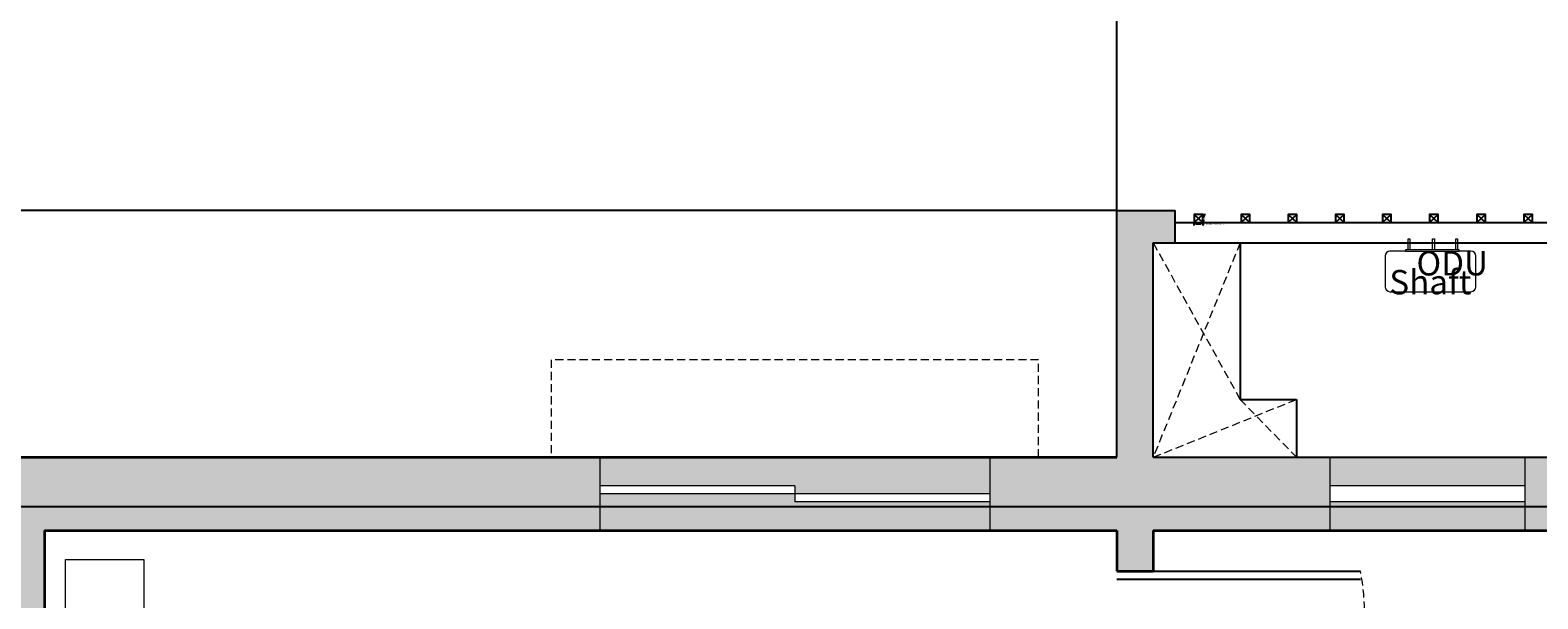
# Model space of a CAD drawing. Units: inches. Extents: x 1693 to 2974, y 2201 to 2965.
# Tile 6 of 24: x 1790 to 1976, y 2689 to 2759. Entities that reach past the tile are written whole.
import ezdxf

# ---------------------------------------------------------------- set-up
doc = ezdxf.new("R2010")
doc.units = ezdxf.units.IN
doc.header["$LTSCALE"] = 2
doc.header["$MEASUREMENT"] = 0
doc.linetypes.add('HIDDEN', pattern=[0.375, 0.25, -0.125])
for name, color, linetype, lineweight in [('A-ANNO-DIMS', 2, 'Continuous', 18), ('A-ANNO-TEXT', 7, 'Continuous', 13), ('A-DOOR', 3, 'Continuous', 25), ('A-DOOR-SWNG', 3, 'HIDDEN', 13), ('A-FLOR-SHFT', 7, 'Continuous', 25), ('A-FLOR-SHFT-HIDN', 8, 'HIDDEN', 13), ('A-FURN', 8, 'Continuous', 18), ('A-GLAZ', 4, 'Continuous', 18), ('A-GLAZ-OVHD', 8, 'HIDDEN', 13), ('A-WALL', 7, 'Continuous', 35), ('M-HVAC-EQPM', 151, 'Continuous', 18)]:
    doc.layers.add(name, color=color, linetype=linetype, lineweight=lineweight)
doc.layers.add('A-GLAZ-PATT', color=141, linetype='Continuous', lineweight=13, true_color=0xadddf7)
doc.layers.add('A-WALL-PATT', color=251, linetype='Continuous', lineweight=13, true_color=0x636466)
doc.styles.get("Standard").update_dxf_attribs({"font": 'arial.ttf'})
doc.dimstyles.get("Standard").update_dxf_attribs({"dimtxt": 0.18, "dimasz": 0.18, "dimexe": 0.18, "dimexo": 0.0625, "dimgap": 0.09, "dimtad": 0, "dimtih": 1, "dimtoh": 1, "dimdec": 1, "dimzin": 0, "dimdsep": 46, "dimlunit": 3, "dimtxsty": 'Standard', "dimcen": 0.09, "dimadec": 0, "dimazin": 0, "dimtfac": 1, "dimtdec": 1, "dimtofl": 0, "dimtmove": 0, "dimatfit": 3, "dimfxl": 1, "dimtolj": 1, "dimtzin": 0, "dimarcsym": 0})

# ---------------------------------------------------------------- blocks, each defined once
blk = doc.blocks.new('NIGHTSTAND')
at = {"ltscale": 2}
blk.add_lwpolyline([(11.51, 0), (0, 0), (0, 9.62), (11.51, 9.62)], close=True, dxfattribs=at)
blk = doc.blocks.new('SHAFT-GUARD-POST-A')
for p, q in [((1.07, 1.01), (0, 0)), ((0, 1.01), (1.07, 0))]:
    blk.add_line(p, q)
blk.add_lwpolyline([(0, 0), (1.07, 0), (1.07, 1.01), (0, 1.01)], close=True)
blk = doc.blocks.new('WINDOW-HOOD-60IN')
at = {"ltscale": 2}
for p, q in [((6, 12), (0, 12)), ((0, 12), (0, 0)), ((60, 12), (6, 12)), ((60, 0), (60, 12)), ((54, 0), (60, 0))]:
    blk.add_line(p, q, dxfattribs=at)
blk = doc.blocks.new('*D31')
at = {"layer": 'A-ANNO-DIMS', "color": 0, "lineweight": -2, "ltscale": 2, "transparency": 16777216}
for p, q in [((1933.25, 2735.65), (1933.25, 2735.38)), ((1934.32, 2735.65), (1934.32, 2735.38)), ((1933.43, 2735.56), (1934.14, 2735.56)), ((1934.32, 2735.56), (1934.5, 2735.56))]:
    blk.add_line(p, q, dxfattribs=at)
at = {"layer": 'A-ANNO-DIMS', "color": 0, "ltscale": 2, "transparency": 16777216}
for points in [[(1933.43, 2735.59), (1933.43, 2735.53), (1933.25, 2735.56)], [(1934.14, 2735.59), (1934.14, 2735.53), (1934.32, 2735.56)]]:
    blk.add_solid(points, dxfattribs=at)
at = {"layer": 'Defpoints', "color": 0, "ltscale": 2, "transparency": 16777216}
for p in [(1933.25, 2735.72), (1934.32, 2735.72), (1934.32, 2735.56)]:
    blk.add_point(p, dxfattribs=at)
at = {"layer": 'A-ANNO-DIMS', "color": 0, "ltscale": 2, "transparency": 16777216, "insert": (1935.94, 2735.56), "char_height": 0.18, "attachment_point": 5}
blk.add_mtext('\\A1;GUARD POST A 1 TYP.', dxfattribs=at)
blk = doc.blocks.new('*D32')
at = {"layer": 'A-ANNO-DIMS', "color": 0, "lineweight": -2, "ltscale": 2, "transparency": 16777216}
for p, q in [((1934.38, 2736.73), (1934.66, 2736.73)), ((1934.38, 2735.72), (1934.66, 2735.72)), ((1934.48, 2736.55), (1934.48, 2736.4)), ((1934.48, 2735.9), (1934.48, 2736.04))]:
    blk.add_line(p, q, dxfattribs=at)
at = {"layer": 'A-ANNO-DIMS', "color": 0, "ltscale": 2, "transparency": 16777216}
for points in [[(1934.45, 2736.55), (1934.51, 2736.55), (1934.48, 2736.73)], [(1934.45, 2735.9), (1934.51, 2735.9), (1934.48, 2735.72)]]:
    blk.add_solid(points, dxfattribs=at)
at = {"layer": 'Defpoints', "color": 0, "ltscale": 2, "transparency": 16777216}
for p in [(1934.32, 2736.73), (1934.32, 2735.72), (1934.48, 2736.73)]:
    blk.add_point(p, dxfattribs=at)
at = {"layer": 'A-ANNO-DIMS', "color": 0, "ltscale": 2, "transparency": 16777216, "insert": (1934.48, 2736.22), "char_height": 0.18, "attachment_point": 5}
blk.add_mtext('\\A1;1 TYP.', dxfattribs=at)
blk = doc.blocks.new('*D81')
at = {"layer": 'A-ANNO-DIMS', "color": 0, "lineweight": -2, "ltscale": 2, "transparency": 16777216}
for p, q in [((1752.34, 2553.91), (1752.34, 2964.96)), ((1752.52, 2964.78), (2332.94, 2964.78)), ((2914.06, 2964.78), (2333.64, 2964.78)), ((2914.24, 2754.97), (2914.24, 2964.96))]:
    blk.add_line(p, q, dxfattribs=at)
at = {"layer": 'A-ANNO-DIMS', "color": 0, "ltscale": 2, "transparency": 16777216}
for points in [[(1752.52, 2964.81), (1752.52, 2964.75), (1752.34, 2964.78)], [(2914.06, 2964.81), (2914.06, 2964.75), (2914.24, 2964.78)]]:
    blk.add_solid(points, dxfattribs=at)
at = {"layer": 'Defpoints', "color": 0, "ltscale": 2, "transparency": 16777216}
for p in [(2914.24, 2964.78), (2914.24, 2754.9), (1752.34, 2553.84)]:
    blk.add_point(p, dxfattribs=at)
at = {"layer": 'A-ANNO-DIMS', "color": 0, "ltscale": 2, "transparency": 16777216, "insert": (2333.29, 2964.78), "char_height": 0.18, "attachment_point": 5}
blk.add_mtext('\\A1;1162', dxfattribs=at)
blk = doc.blocks.new('*D82')
at = {"layer": 'A-ANNO-DIMS', "color": 0, "lineweight": -2, "ltscale": 2, "transparency": 16777216}
for p, q in [((2615.67, 2906.08), (1693.46, 2906.08)), ((1693.64, 2905.9), (1693.64, 2582.94)), ((1693.64, 2259.62), (1693.64, 2582.58)), ((2096.17, 2259.44), (1693.46, 2259.44))]:
    blk.add_line(p, q, dxfattribs=at)
at = {"layer": 'A-ANNO-DIMS', "color": 0, "ltscale": 2, "transparency": 16777216}
for points in [[(1693.61, 2905.9), (1693.67, 2905.9), (1693.64, 2906.08)], [(1693.61, 2259.62), (1693.67, 2259.62), (1693.64, 2259.44)]]:
    blk.add_solid(points, dxfattribs=at)
at = {"layer": 'Defpoints', "color": 0, "ltscale": 2, "transparency": 16777216}
for p in [(1693.64, 2906.08), (2615.74, 2906.08), (2096.24, 2259.44)]:
    blk.add_point(p, dxfattribs=at)
at = {"layer": 'A-ANNO-DIMS', "color": 0, "ltscale": 2, "transparency": 16777216, "insert": (1693.64, 2582.76), "char_height": 0.18, "attachment_point": 5}
blk.add_mtext('\\A1;646.6', dxfattribs=at)
blk = doc.blocks.new('*D88')
at = {"layer": 'A-ANNO-DIMS', "color": 0, "lineweight": -2, "ltscale": 2, "transparency": 16777216}
for p, q in [((2479.17, 2700.75), (1693.46, 2700.75)), ((1693.64, 2700.57), (1693.64, 2666.44)), ((1693.64, 2631.93), (1693.64, 2666.07)), ((2479.17, 2631.75), (1693.46, 2631.75))]:
    blk.add_line(p, q, dxfattribs=at)
at = {"layer": 'A-ANNO-DIMS', "color": 0, "ltscale": 2, "transparency": 16777216}
for points in [[(1693.61, 2700.57), (1693.67, 2700.57), (1693.64, 2700.75)], [(1693.61, 2631.93), (1693.67, 2631.93), (1693.64, 2631.75)]]:
    blk.add_solid(points, dxfattribs=at)
at = {"layer": 'Defpoints', "color": 0, "ltscale": 2, "transparency": 16777216}
for p in [(1693.64, 2700.75), (2479.24, 2700.75), (2479.24, 2631.75)]:
    blk.add_point(p, dxfattribs=at)
at = {"layer": 'A-ANNO-DIMS', "color": 0, "ltscale": 2, "transparency": 16777216, "insert": (1693.64, 2666.25), "char_height": 0.18, "attachment_point": 5}
blk.add_mtext('\\A1;69', dxfattribs=at)
blk = doc.blocks.new('*D102')
at = {"layer": 'A-ANNO-DIMS', "color": 0, "lineweight": -2, "ltscale": 2, "transparency": 16777216}
for p, q in [((1782.74, 2706.91), (1782.74, 2964.96)), ((1782.92, 2964.78), (1852.97, 2964.78)), ((1923.56, 2964.78), (1853.5, 2964.78)), ((1923.74, 2706.91), (1923.74, 2964.96))]:
    blk.add_line(p, q, dxfattribs=at)
at = {"layer": 'A-ANNO-DIMS', "color": 0, "ltscale": 2, "transparency": 16777216}
for points in [[(1782.92, 2964.81), (1782.92, 2964.75), (1782.74, 2964.78)], [(1923.56, 2964.81), (1923.56, 2964.75), (1923.74, 2964.78)]]:
    blk.add_solid(points, dxfattribs=at)
at = {"layer": 'Defpoints', "color": 0, "ltscale": 2, "transparency": 16777216}
for p in [(1923.74, 2964.78), (1782.74, 2706.84), (1923.74, 2706.84)]:
    blk.add_point(p, dxfattribs=at)
at = {"layer": 'A-ANNO-DIMS', "color": 0, "ltscale": 2, "transparency": 16777216, "insert": (1853.24, 2964.78), "char_height": 0.18, "attachment_point": 5}
blk.add_mtext('\\A1;141', dxfattribs=at)
blk = doc.blocks.new('*D103')
at = {"layer": 'A-ANNO-DIMS', "color": 0, "lineweight": -2, "ltscale": 2, "transparency": 16777216}
for p, q in [((1923.74, 2737.28), (1923.74, 2964.96)), ((1923.92, 2964.78), (1959.52, 2964.78)), ((1995.56, 2964.78), (1959.95, 2964.78)), ((1995.74, 2737.28), (1995.74, 2964.96))]:
    blk.add_line(p, q, dxfattribs=at)
at = {"layer": 'A-ANNO-DIMS', "color": 0, "ltscale": 2, "transparency": 16777216}
for points in [[(1923.92, 2964.81), (1923.92, 2964.75), (1923.74, 2964.78)], [(1995.56, 2964.81), (1995.56, 2964.75), (1995.74, 2964.78)]]:
    blk.add_solid(points, dxfattribs=at)
at = {"layer": 'Defpoints', "color": 0, "ltscale": 2, "transparency": 16777216}
for p in [(1995.74, 2964.78), (1923.74, 2737.22), (1995.74, 2737.22)]:
    blk.add_point(p, dxfattribs=at)
at = {"layer": 'A-ANNO-DIMS', "color": 0, "ltscale": 2, "transparency": 16777216, "insert": (1959.74, 2964.78), "char_height": 0.18, "attachment_point": 5}
blk.add_mtext('\\A1;72', dxfattribs=at)
blk = doc.blocks.new('*D105')
at = {"layer": 'A-ANNO-DIMS', "color": 0, "lineweight": -2, "ltscale": 2, "transparency": 16777216}
for p, q in [((1923.67, 2737.22), (1693.46, 2737.22)), ((1693.64, 2737.04), (1693.64, 2722.21)), ((1693.64, 2707.02), (1693.64, 2721.85)), ((1923.67, 2706.84), (1693.46, 2706.84))]:
    blk.add_line(p, q, dxfattribs=at)
at = {"layer": 'A-ANNO-DIMS', "color": 0, "ltscale": 2, "transparency": 16777216}
for points in [[(1693.61, 2737.04), (1693.67, 2737.04), (1693.64, 2737.22)], [(1693.61, 2707.02), (1693.67, 2707.02), (1693.64, 2706.84)]]:
    blk.add_solid(points, dxfattribs=at)
at = {"layer": 'Defpoints', "color": 0, "ltscale": 2, "transparency": 16777216}
for p in [(1693.64, 2737.22), (1923.74, 2737.22), (1923.74, 2706.84)]:
    blk.add_point(p, dxfattribs=at)
at = {"layer": 'A-ANNO-DIMS', "color": 0, "ltscale": 2, "transparency": 16777216, "insert": (1693.64, 2722.03), "char_height": 0.18, "attachment_point": 5}
blk.add_mtext('\\A1;30.37', dxfattribs=at)

msp = doc.modelspace()

# ---------------------------------------------------------------- hatches: boundary and pattern name
at = {"layer": 'A-GLAZ-PATT', "ltscale": 2}
h = msp.add_hatch(color=256, dxfattribs=at)
h.dxf.hatch_style = 1
h.paths.add_polyline_path([(2656.9702, 2338.2547), (2632.9702, 2338.2547), (2632.9702, 2339.2547), (2608.9702, 2339.2547), (2608.9702, 2334.7547), (2656.9702, 2334.7547)])
h.paths.add_polyline_path([(2656.9702, 2343.7547), (2608.9702, 2343.7547), (2608.9702, 2340.2547), (2632.9702, 2340.2547), (2632.9702, 2339.2547), (2656.9702, 2339.2547)])
h.paths.add_polyline_path([(2775.7544, 2338.2547), (2751.7544, 2338.2547), (2751.7544, 2334.7547), (2775.7544, 2334.7547)])
h.paths.add_polyline_path([(2775.7544, 2343.7547), (2751.7544, 2343.7547), (2751.7544, 2340.2547), (2775.7544, 2340.2547)])
h.paths.add_polyline_path([(2897.7363, 2568.7999), (2893.2363, 2568.7999), (2893.2363, 2520.7999), (2896.7363, 2520.7999), (2896.7363, 2544.7999), (2897.7363, 2544.7999)])
h.paths.add_polyline_path([(2902.2363, 2568.7999), (2898.7363, 2568.7999), (2898.7363, 2544.7999), (2897.7363, 2544.7999), (2897.7363, 2520.7999), (2902.2363, 2520.7999)])
h.paths.add_polyline_path([(2902.2363, 2637.7547), (2898.7363, 2637.7547), (2898.7363, 2613.7547), (2902.2363, 2613.7547)])
h.paths.add_polyline_path([(2896.7363, 2637.7547), (2893.2363, 2637.7547), (2893.2363, 2613.7547), (2896.7363, 2613.7547)])
h.paths.add_polyline_path([(2902.2363, 2748.903), (2899.0477, 2748.903), (2899.0477, 2724.903), (2898.0477, 2724.903), (2898.0477, 2700.903), (2902.2363, 2700.903)])
h.paths.add_polyline_path([(2898.0477, 2748.903), (2893.2363, 2748.903), (2893.2363, 2700.903), (2897.0477, 2700.903), (2897.0477, 2724.903), (2898.0477, 2724.903)])
h.paths.add_polyline_path([(2851.2363, 2846.2547), (2803.2363, 2846.2547), (2803.2363, 2842.7547), (2827.2363, 2842.7547), (2827.2363, 2841.7547), (2851.2363, 2841.7547)])
h.paths.add_polyline_path([(2851.2363, 2840.7547), (2827.2363, 2840.7547), (2827.2363, 2841.7547), (2803.2363, 2841.7547), (2803.2363, 2837.2547), (2851.2363, 2837.2547)])
h.paths.add_polyline_path([(2578.2363, 2846.2547), (2530.2363, 2846.2547), (2530.2363, 2842.7547), (2554.2363, 2842.7547), (2554.2363, 2841.7547), (2578.2363, 2841.7547)])
h.paths.add_polyline_path([(2578.2363, 2840.7547), (2554.2363, 2840.7547), (2554.2363, 2841.7547), (2530.2363, 2841.7547), (2530.2363, 2837.2547), (2578.2363, 2837.2547)])
h.paths.add_polyline_path([(2732.7363, 2812.7547), (2705.1363, 2812.7547), (2705.1363, 2811.7547), (2676.3363, 2811.7547), (2676.3363, 2812.7547), (2648.7363, 2812.7547), (2648.7363, 2808.2547), (2732.7363, 2808.2547)])
h.paths.add_polyline_path([(2732.7363, 2817.2547), (2648.7363, 2817.2547), (2648.7363, 2813.7547), (2676.3363, 2813.7547), (2676.3363, 2812.7547), (2705.1363, 2812.7547), (2705.1363, 2813.7547), (2732.7363, 2813.7547)])
h.paths.add_polyline_path([(2488.2363, 2695.8203), (2484.7878, 2695.8203), (2484.7878, 2671.8203), (2488.2363, 2671.8203)])
h.paths.add_polyline_path([(2482.7878, 2695.8203), (2479.2363, 2695.8203), (2479.2363, 2671.8203), (2482.7878, 2671.8203)])
h.paths.add_polyline_path([(2488.2363, 2572.4371), (2484.7363, 2572.4371), (2484.7363, 2541.4371), (2483.7363, 2541.4371), (2483.7363, 2512.4371), (2488.2363, 2512.4371)])
h.paths.add_polyline_path([(2482.7363, 2541.4371), (2483.7363, 2541.4371), (2483.7363, 2572.4371), (2479.2363, 2572.4371), (2479.2363, 2512.4371), (2482.7363, 2512.4371)])
h.paths.add_polyline_path([(2248.9863, 2706.8449), (2190.9863, 2706.8449), (2190.9863, 2703.3449), (2219.9863, 2703.3449), (2219.9863, 2702.3449), (2248.9863, 2702.3449)])
h.paths.add_polyline_path([(2248.9863, 2701.3449), (2219.9863, 2701.3449), (2219.9863, 2702.3449), (2190.9863, 2702.3449), (2190.9863, 2697.8449), (2248.9863, 2697.8449)])
h.paths.add_polyline_path([(2151.9207, 2293.3449), (2127.9207, 2293.3449), (2127.9207, 2289.8449), (2151.9207, 2289.8449)])
h.paths.add_polyline_path([(2151.9207, 2298.8449), (2127.9207, 2298.8449), (2127.9207, 2295.3449), (2151.9207, 2295.3449)])
h.paths.add_polyline_path([(2084.023, 2293.3449), (2066.023, 2293.3449), (2066.023, 2294.3449), (2048.023, 2294.3449), (2048.023, 2289.8449), (2084.023, 2289.8449)])
h.paths.add_polyline_path([(2084.023, 2298.8449), (2048.023, 2298.8449), (2048.023, 2295.3449), (2066.023, 2295.3449), (2066.023, 2294.3449), (2084.023, 2294.3449)])
h.paths.add_polyline_path([(1966.0781, 2293.3449), (1948.0781, 2293.3449), (1948.0781, 2294.3449), (1930.0781, 2294.3449), (1930.0781, 2289.8449), (1966.0781, 2289.8449)])
h.paths.add_polyline_path([(1966.0781, 2298.8449), (1930.0781, 2298.8449), (1930.0781, 2295.3449), (1948.0781, 2295.3449), (1948.0781, 2294.3449), (1966.0781, 2294.3449)])
h.paths.add_polyline_path([(1787.2363, 2403.1922), (1782.7363, 2403.1922), (1782.7363, 2355.1922), (1786.2363, 2355.1922), (1786.2363, 2379.1922), (1787.2363, 2379.1922)])
h.paths.add_polyline_path([(1791.7363, 2403.1922), (1788.2363, 2403.1922), (1788.2363, 2379.1922), (1787.2363, 2379.1922), (1787.2363, 2355.1922), (1791.7363, 2355.1922)])
h.paths.add_polyline_path([(1786.2363, 2477.5455), (1782.7363, 2477.5455), (1782.7363, 2453.5455), (1786.2363, 2453.5455)])
h.paths.add_polyline_path([(1791.7363, 2477.5455), (1788.2363, 2477.5455), (1788.2363, 2453.5455), (1791.7363, 2453.5455)])
h.paths.add_polyline_path([(1786.2363, 2621.6433), (1782.7363, 2621.6433), (1782.7363, 2585.6433), (1786.2363, 2585.6433)])
h.paths.add_polyline_path([(1791.7363, 2621.6433), (1788.2363, 2621.6433), (1788.2363, 2585.6433), (1791.7363, 2585.6433)])
h.paths.add_polyline_path([(1908.1286, 2706.8449), (1860.1286, 2706.8449), (1860.1286, 2703.3449), (1884.1286, 2703.3449), (1884.1286, 2702.3449), (1908.1286, 2702.3449)])
h.paths.add_polyline_path([(1908.1286, 2701.3449), (1884.1286, 2701.3449), (1884.1286, 2702.3449), (1860.1286, 2702.3449), (1860.1286, 2697.8449), (1908.1286, 2697.8449)])
h.paths.add_polyline_path([(1973.9863, 2706.8449), (1949.9863, 2706.8449), (1949.9863, 2703.3449), (1973.9863, 2703.3449)])
h.paths.add_polyline_path([(1973.9863, 2701.3449), (1949.9863, 2701.3449), (1949.9863, 2697.8449), (1973.9863, 2697.8449)])
h.paths.add_polyline_path([(2112.7363, 2690.3449), (2028.7363, 2690.3449), (2028.7363, 2686.8449), (2056.3363, 2686.8449), (2056.3363, 2685.8449), (2085.1363, 2685.8449), (2085.1363, 2686.8449), (2112.7363, 2686.8449)])
h.paths.add_polyline_path([(2112.7363, 2685.8449), (2085.1363, 2685.8449), (2085.1363, 2684.8449), (2056.3363, 2684.8449), (2056.3363, 2685.8449), (2028.7363, 2685.8449), (2028.7363, 2681.3449), (2112.7363, 2681.3449)])
h.paths.add_polyline_path([(2422.7363, 2640.7547), (2350.7363, 2640.7547), (2350.7363, 2637.2547), (2386.7363, 2637.2547), (2386.7363, 2636.2547), (2422.7363, 2636.2547)])
h.paths.add_polyline_path([(2422.7363, 2635.2547), (2386.7363, 2635.2547), (2386.7363, 2636.2547), (2350.7363, 2636.2547), (2350.7363, 2631.7547), (2422.7363, 2631.7547)])
at = {"layer": 'A-WALL-PATT', "ltscale": 2}
h = msp.add_hatch(color=256, dxfattribs=at)
h.dxf.hatch_style = 1
h.paths.add_polyline_path([(1928.2363, 2733.2161), (1930.9384, 2733.2161), (1930.9384, 2737.2161), (1923.7363, 2737.2161), (1923.7363, 2706.8449), (1908.1286, 2706.8449), (1908.1286, 2697.8449), (1923.7363, 2697.8449), (1923.7363, 2692.8449), (1928.2363, 2692.8449), (1928.2363, 2697.8449), (1949.9863, 2697.8449), (1949.9863, 2706.8449), (1928.2363, 2706.8449)])
h.paths.add_polyline_path([(2004.7363, 2737.2161), (1995.7363, 2737.2161), (1995.7363, 2706.8449), (1985.6374, 2706.8449), (1973.9863, 2706.8449), (1973.9863, 2697.8449), (2000.2363, 2697.8449), (2000.2363, 2686.5348), (2000.3613, 2686.5348), (2000.3613, 2667.0432), (2000.2363, 2601.8449), (1928.2363, 2601.8449), (1928.2363, 2662.8449), (1923.7363, 2662.8449), (1923.7363, 2595.3449), (1928.2363, 2595.3449), (1928.2363, 2597.3449), (2004.7363, 2597.3449), (2004.7363, 2681.3449), (2012.7814, 2681.3449), (2028.7363, 2681.3449), (2028.7363, 2690.3449), (2004.7363, 2690.3449)])
h.paths.add_polyline_path([(2190.9863, 2706.8449), (2184.9863, 2706.8449), (2145.7363, 2706.8449), (2145.7363, 2765.3449), (2145.7363, 2774.5394), (2136.7363, 2774.5394), (2136.7363, 2756.3449), (2136.7363, 2690.3449), (2112.7363, 2690.3449), (2112.7363, 2681.3449), (2136.7363, 2681.3449), (2136.7363, 2597.3449), (2141.2363, 2597.3449), (2141.2363, 2697.8449), (2190.9863, 2697.8449)])
h.paths.add_polyline_path([(1860.1286, 2706.8449), (1782.7363, 2706.8449), (1782.7363, 2621.6433), (1791.7363, 2621.6433), (1791.7363, 2697.8449), (1860.1286, 2697.8449)])
h.paths.add_polyline_path([(1791.7363, 2585.6433), (1782.7363, 2585.6433), (1782.7363, 2562.8449), (1782.7363, 2553.8449), (1752.3363, 2553.8449), (1752.3363, 2544.2586), (1756.3363, 2544.2586), (1756.3363, 2549.3449), (1782.7363, 2549.3449), (1782.7363, 2489.2404), (1782.7363, 2477.5455), (1791.7363, 2477.5455), (1791.7363, 2493.5991), (1791.6113, 2493.5991), (1791.6113, 2513.0907), (1791.6824, 2533.7198, -0.94742783), (1791.7363, 2534.7168), (1791.7363, 2549.3449), (1863.7363, 2549.3449), (1863.7363, 2513.3449), (1866.7363, 2513.3449), (1866.7363, 2549.3449), (1924.7363, 2549.3449), (1924.7363, 2447.3449), (1924.7363, 2442.8449), (1933.7363, 2442.8449), (1933.7363, 2447.3449), (1928.2363, 2447.3449), (1928.2363, 2559.3449), (1923.7363, 2559.3449), (1923.7363, 2553.8449), (1791.7363, 2553.8449), (1791.7363, 2562.8449)])
h.paths.add_polyline_path([(1791.7363, 2442.8449), (1866.7363, 2442.8449), (1866.7363, 2447.3449), (1866.7363, 2483.3449), (1863.7363, 2483.3449), (1863.7363, 2447.3449), (1791.7363, 2447.3449), (1791.7363, 2453.5455), (1782.7363, 2453.5455), (1782.7363, 2447.3449), (1756.3363, 2447.3449), (1756.3363, 2455.7126), (1752.3363, 2455.7126), (1752.3363, 2442.8449), (1782.7363, 2442.8449), (1782.7363, 2403.1922), (1791.7363, 2403.1922)])
h.paths.add_polyline_path([(1930.0781, 2298.8449), (1791.7363, 2298.8449), (1791.7363, 2355.1922), (1782.7363, 2355.1922), (1782.7363, 2289.8449), (1930.0781, 2289.8449)])
h.paths.add_polyline_path([(2624.7363, 2883.2547), (2624.7363, 2902.6165), (2624.7363, 2906.0761), (2615.7363, 2906.0761), (2615.7363, 2892.2547), (2615.7363, 2846.2547), (2578.2363, 2846.2547), (2578.2363, 2837.2547), (2620.2363, 2837.2547), (2620.2363, 2743.2547), (2624.7363, 2743.2547), (2624.7363, 2808.2547), (2648.7363, 2808.2547), (2648.7363, 2817.2547), (2624.7363, 2817.2547)])
h.paths.add_polyline_path([(2530.2363, 2846.2547), (2479.2363, 2846.2547), (2479.2363, 2695.8203), (2488.2363, 2695.8203), (2488.2363, 2700.7547), (2567.2363, 2700.7547), (2567.2363, 2705.2547), (2488.2363, 2705.2547), (2488.2363, 2837.2547), (2530.2363, 2837.2547)])
h.paths.add_polyline_path([(2488.2363, 2487.7547), (2630.2363, 2487.7547, -0.00990191), (2630.2363, 2489.0322), (2630.2363, 2492.2547), (2488.2363, 2492.2547), (2488.2363, 2512.4371), (2479.2363, 2512.4371), (2479.2363, 2334.7547), (2608.9702, 2334.7547), (2608.9702, 2343.7547), (2488.2363, 2343.7547)])
h.paths.add_polyline_path([(2751.7544, 2343.7547), (2672.7363, 2343.7547), (2672.7363, 2409.7547), (2674.7363, 2409.7547), (2674.7363, 2413.7547), (2672.7363, 2413.7547), (2672.7363, 2487.7547), (2732.7363, 2487.7547), (2732.7363, 2413.7547), (2704.7363, 2413.7547), (2704.7363, 2409.7547), (2784.7363, 2409.7547), (2784.7363, 2343.7547), (2775.7544, 2343.7547), (2775.7544, 2334.7547), (2902.2363, 2334.7547), (2902.2363, 2520.7999), (2893.2363, 2520.7999), (2893.2363, 2413.7547), (2856.0145, 2413.7547), (2856.0145, 2409.7547), (2893.2363, 2409.7547), (2893.2363, 2343.7547), (2789.2363, 2343.7547), (2789.2363, 2409.7547), (2819.2363, 2409.7547), (2826.0145, 2409.7547), (2826.0145, 2413.7547), (2789.2363, 2413.7547), (2789.2363, 2492.2547), (2784.7363, 2492.2547), (2784.7363, 2413.7547), (2736.7363, 2413.7547), (2736.7363, 2492.2547), (2672.7363, 2492.2547), (2666.2363, 2492.2547), (2666.2363, 2487.7547), (2668.2363, 2487.7547), (2668.2363, 2343.7547), (2656.9702, 2343.7547), (2656.9702, 2334.7547), (2662.9702, 2334.7547), (2751.7544, 2334.7547)])
h.paths.add_polyline_path([(2902.2363, 2613.7547), (2893.2363, 2613.7547), (2893.2363, 2589.7547), (2785.2363, 2589.7547), (2785.2363, 2661.7547), (2790.2363, 2661.7547), (2790.2363, 2665.2547), (2761.2363, 2665.2547), (2761.2363, 2667.2547), (2756.7363, 2667.2547), (2756.7363, 2661.7547), (2781.2363, 2661.7547), (2781.2363, 2585.7547), (2893.2363, 2585.7547), (2893.2363, 2568.7999), (2902.2363, 2568.7999)])
h.paths.add_polyline_path([(2488.2363, 2671.8203), (2479.2363, 2671.8203), (2479.2363, 2645.2547), (2479.2363, 2623.4598), (2488.2363, 2623.4598), (2488.2363, 2636.2547), (2624.7363, 2636.2547), (2624.7363, 2640.7547), (2603.7363, 2640.7547), (2603.7363, 2700.7547), (2624.7363, 2700.7547), (2624.7363, 2707.2547), (2620.2363, 2707.2547), (2620.2363, 2705.2547), (2597.2363, 2705.2547), (2597.2363, 2700.7547), (2599.2363, 2700.7547), (2599.2363, 2640.7547), (2488.2363, 2640.7547)])
h.paths.add_polyline_path([(2761.2363, 2837.2547), (2803.2363, 2837.2547), (2803.2363, 2846.2547), (2797.2363, 2846.2547), (2765.7363, 2846.2547), (2756.7363, 2846.2547), (2756.7363, 2817.2547), (2732.7363, 2817.2547), (2732.7363, 2808.2547), (2756.7363, 2808.2547), (2756.7363, 2703.2547), (2761.2363, 2703.2547)])
h.paths.add_polyline_path([(2739.7489, 2433.1234), (2786.9181, 2433.1234), (2786.9181, 2455.5122), (2739.7489, 2455.5122)], flags=25)

# ---------------------------------------------------------------- linework, layer by layer
at = {"layer": 'A-DOOR', "ltscale": 2}
for p, q in [((1923.7363, 2692.8449), (1953.7363, 2692.8449)), ((1923.7363, 2691.8449), (1953.7363, 2691.8449))]:
    msp.add_line(p, q, dxfattribs=at)
at = {"layer": 'A-DOOR-SWNG', "ltscale": 2}
msp.add_arc((1929.1915, 2687.8705), 25.0438, 267.814245, 11.456682, dxfattribs=at)
at = {"layer": 'A-FLOR-SHFT'}
for p, q in [((1923.7363, 2706.8449), (1923.7363, 2737.2161)), ((1923.7363, 2737.2161), (1930.9384, 2737.2161)), ((1930.9384, 2733.2161), (1930.9384, 2737.2161)), ((1930.9384, 2735.7161), (1995.7363, 2735.7161)), ((1928.2363, 2706.8449), (1928.2363, 2733.2161)), ((1928.2363, 2733.2161), (1995.7363, 2733.2161)), ((1938.9241, 2733.2161), (1938.9241, 2713.9573)), ((1938.9241, 2713.9573), (1945.8772, 2713.9573)), ((1945.8772, 2713.9573), (1945.8772, 2706.8449)), ((1928.2363, 2706.8449), (1995.7363, 2706.8449))]:
    msp.add_line(p, q, dxfattribs=at)
at = {"layer": 'A-FLOR-SHFT-HIDN', "ltscale": 2}
for p, q in [((1928.2363, 2733.2161), (1938.9241, 2713.9573)), ((1938.9241, 2733.2161), (1928.2363, 2706.8449)), ((1928.2363, 2706.8449), (1945.8772, 2713.9573)), ((1938.9241, 2713.9573), (1945.8772, 2706.8449))]:
    msp.add_line(p, q, dxfattribs=at)
at = {"layer": 'A-GLAZ', "ltscale": 2}
for p, q in [((1860.1286, 2706.8449), (1860.1286, 2697.8449)), ((1908.1286, 2706.8449), (1908.1286, 2697.8449)), ((1949.9863, 2706.8449), (1949.9863, 2697.8449)), ((1973.9863, 2706.8449), (1973.9863, 2697.8449)), ((1884.1286, 2703.3449), (1860.1286, 2703.3449)), ((1908.1286, 2702.3449), (1860.1286, 2702.3449)), ((1884.1286, 2703.3449), (1884.1286, 2701.3449)), ((1973.9863, 2703.3449), (1949.9863, 2703.3449)), ((1908.1286, 2701.3449), (1884.1286, 2701.3449)), ((1973.9863, 2701.3449), (1949.9863, 2701.3449))]:
    msp.add_line(p, q, dxfattribs=at)
at = {"layer": 'A-WALL'}
for p, q in [((1782.7363, 2706.8449), (1923.7363, 2706.8449)), ((1791.7363, 2697.8449), (1923.7363, 2697.8449)), ((1791.7363, 2697.8449), (1791.7363, 2562.8449)), ((1923.7363, 2697.8449), (1923.7363, 2692.8449)), ((1928.2363, 2697.8449), (1928.2363, 2692.8449)), ((1928.2363, 2697.8449), (2000.2363, 2697.8449)), ((1923.7363, 2692.8449), (1928.2363, 2692.8449))]:
    msp.add_line(p, q, dxfattribs=at)
at = {"layer": 'M-HVAC-EQPM'}
for p, q in [((1965.6931, 2732.3748), (1959.2669, 2732.3748)), ((1959.2669, 2732.3748), (1959.2669, 2732.2155)), ((1959.2669, 2732.2155), (1965.8755, 2732.2155)), ((1965.8755, 2732.3748), (1965.6931, 2732.3748)), ((1965.8755, 2732.2155), (1965.8755, 2732.3748))]:
    msp.add_line(p, q, dxfattribs=at)
msp.add_lwpolyline([(1959.2669, 2732.2155), (1958.7113, 2732.2155), (1957.3682, 2732.2155, 0.41421356), (1956.7682, 2731.6155), (1956.7682, 2727.8162, 0.41421356), (1957.3682, 2727.2162), (1967.348, 2727.2162, 0.41421356), (1967.948, 2727.8162), (1967.948, 2731.6155, 0.41421356), (1967.348, 2732.2155), (1965.8755, 2732.2155)], format="xyb", dxfattribs=at)
for points in [[(1959.5999, 2733.7277), (1959.8175, 2733.7277), (1959.8175, 2732.3748), (1959.5999, 2732.3748)], [(1962.6223, 2733.7277), (1962.8399, 2733.7277), (1962.8399, 2732.3748), (1962.6223, 2732.3748)], [(1965.4754, 2733.7277), (1965.6931, 2733.7277), (1965.6931, 2732.3748), (1965.4754, 2732.3748)]]:
    msp.add_lwpolyline(points, close=True, dxfattribs=at)

# ---------------------------------------------------------------- block references
at = {"layer": 'A-FLOR-SHFT'}
for p in [(1933.252, 2735.716), (1939.052, 2735.716), (1944.852, 2735.716), (1950.652, 2735.716), (1956.452, 2735.716), (1962.252, 2735.716), (1968.052, 2735.716), (1973.852, 2735.716)]:
    msp.add_blockref('SHAFT-GUARD-POST-A', p, dxfattribs=at)
at = {"layer": 'A-FURN', "rotation": 270.0000000000054}
msp.add_blockref('NIGHTSTAND', (1794.3504, 2694.2704), dxfattribs=at)
at = {"layer": 'A-GLAZ-OVHD'}
msp.add_blockref('WINDOW-HOOD-60IN', (1854.129, 2706.845), dxfattribs=at)

# ---------------------------------------------------------------- texts
at = {"layer": 'A-ANNO-TEXT', "ltscale": 2, "char_height": 3, "attachment_point": 1}
for s, insert in [('ODU', (1960.6395, 2732.2155)), ('Shaft', (1957.2931, 2729.8932))]:
    msp.add_mtext_dynamic_manual_height_columns(s, width=108.452746, gutter_width=1, heights=[0], dxfattribs=dict(at, insert=insert))

# ---------------------------------------------------------------- dimensions: what is measured, and where the dimension line sits
at = {"layer": 'A-ANNO-DIMS', "ltscale": 2}
for base, p1, p2, picture, middle in [((2914.2363, 2964.7761), (1752.3363, 2553.8449), (2914.2363, 2754.903), '*D81', (2333.2863, 2964.7761)), ((1923.7363, 2964.7761), (1782.7363, 2706.8449), (1923.7363, 2706.8449), '*D102', (1853.2363, 2964.7761)), ((1995.7363, 2964.7761), (1923.7363, 2737.2161), (1995.7363, 2737.2161), '*D103', (1959.7363, 2964.7761))]:
    dim = msp.add_linear_dim(base=base, p1=p1, p2=p2, dimstyle='Standard', override={"dimdec": 0, "dimlfac": 1, "dimrnd": 0, "dimzin": 0, "dimdsep": 46, "dimlunit": 2}, dxfattribs=at)
    dim.commit()
    dim.dimension.update_dxf_attribs({"geometry": picture, "text_midpoint": middle})
for base, p1, p2, override, picture, middle in [((1693.6363, 2906.0761), (2096.2363, 2259.4449), (2615.7363, 2906.0761), {"dimdec": 1, "dimlfac": 1, "dimrnd": 0, "dimzin": 0, "dimdsep": 46, "dimlunit": 2}, '*D82', (1693.6363, 2582.7605)), ((1693.6363, 2737.2161), (1923.7363, 2706.8449), (1923.7363, 2737.2161), {"dimdec": 2, "dimlfac": 1, "dimrnd": 0, "dimzin": 0, "dimdsep": 46, "dimlunit": 2}, '*D105', (1693.6363, 2722.0305)), ((1693.6363, 2700.7547), (2479.2363, 2631.7547), (2479.2363, 2700.7547), {"dimdec": 0, "dimlfac": 1, "dimrnd": 0, "dimzin": 0, "dimdsep": 46, "dimlunit": 2}, '*D88', (1693.6363, 2666.2547))]:
    dim = msp.add_linear_dim(base=base, p1=p1, p2=p2, angle=90, dimstyle='Standard', override=override, dxfattribs=at)
    dim.commit()
    dim.dimension.update_dxf_attribs({"geometry": picture, "text_midpoint": middle})
dim = msp.add_linear_dim(base=(1934.3175, 2735.5563), p1=(1933.2524, 2735.7161), p2=(1934.3175, 2735.7161), text='GUARD POST A <> TYP.', dimstyle='Standard', override={"dimdec": 0, "dimlfac": 1, "dimrnd": 0, "dimzin": 0, "dimdsep": 46, "dimlunit": 2}, dxfattribs=at)
dim.commit()
dim.dimension.update_dxf_attribs({"geometry": '*D31', "text_midpoint": (1935.9392, 2735.5563)})
dim = msp.add_linear_dim(base=(1934.4773, 2736.728), p1=(1934.3175, 2735.7161), p2=(1934.3175, 2736.728), angle=90, text='<> TYP.', dimstyle='Standard', override={"dimdec": 0, "dimlfac": 1, "dimrnd": 0, "dimzin": 0, "dimdsep": 46, "dimlunit": 2}, dxfattribs=at)
dim.commit()
dim.dimension.update_dxf_attribs({"geometry": '*D32', "text_midpoint": (1934.4773, 2736.2221)})

doc.saveas('drawing.dxf')
